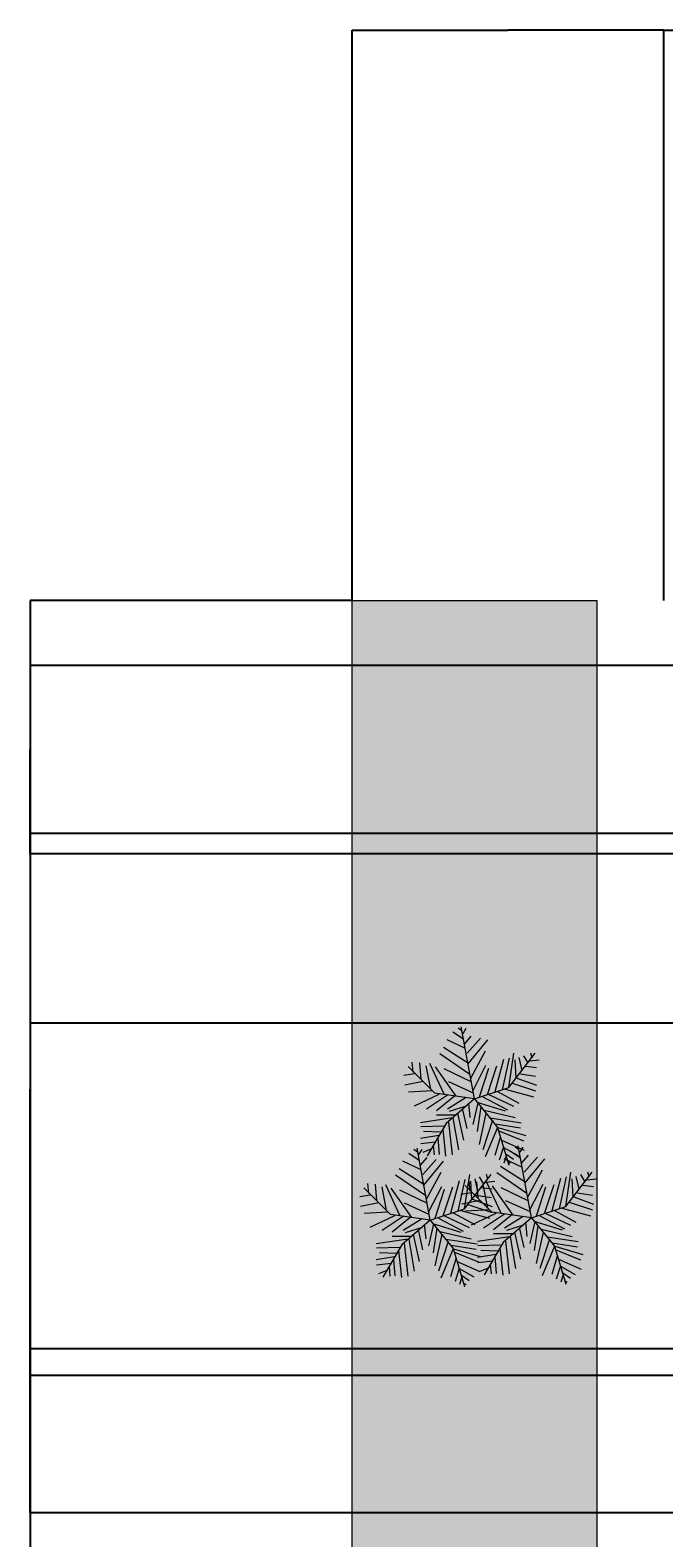
# Model space of a CAD drawing. Units: millimetres. Extents: x -229 to 16545, y -10488 to 4272.
# Tile 4 of 29: x -229 to 2016, y -1067 to 4272. Entities that reach past the tile are written whole.
import ezdxf

# ---------------------------------------------------------------- set-up
doc = ezdxf.new("R2010")
doc.units = ezdxf.units.MM
for name, color, linetype, lineweight in [('A-ANNO-DIMS', 2, 'Continuous', 18), ('L-PLNT-BEDS', 82, 'Continuous', 18), ('L-PLNT-TREE', 80, 'Continuous', 18)]:
    doc.layers.add(name, color=color, linetype=linetype, lineweight=lineweight)
doc.layers.add('L-PLNT-PATT', color=116, linetype='Continuous', lineweight=13, true_color=0x136734)
doc.styles.get("Standard").update_dxf_attribs({"font": 'arial.ttf'})
doc.dimstyles.get("Standard").update_dxf_attribs({"dimtxt": 0.18, "dimasz": 0.18, "dimexe": 0.18, "dimexo": 0.0625, "dimgap": 0.09, "dimtad": 0, "dimtih": 1, "dimtoh": 1, "dimdec": 4, "dimzin": 0, "dimdsep": 46, "dimtxsty": 'Standard', "dimcen": 0.09, "dimadec": 0, "dimazin": 0, "dimtfac": 1, "dimtdec": 4, "dimtofl": 0, "dimtmove": 0, "dimatfit": 3, "dimfxl": 1, "dimtolj": 1, "dimtzin": 0, "dimarcsym": 0})

# ---------------------------------------------------------------- blocks, each defined once
blk = doc.blocks.new('*U18')
for p, q in [((-8.737, 47.138), (-17.069, 52.711)), ((-10.186, 53.64), (-13.084, 55.962)), ((0, 0), (-10.5, 57)), ((-9.099, 51.782), (-6.563, 55.962)), ((-7.65, 43.423), (-2.578, 49.46)), ((-5.839, 35.992), (4.667, 48.067)), ((-5.114, 28.097), (-24.676, 40.636)), ((-7.288, 39.707), (-21.778, 46.673)), ((-5.114, 27.632), (10.463, 46.673)), ((-2.941, 16.486), (8.652, 37.85)), ((27, 9), (48, 36)), ((27.127, 9.056), (31.112, 35.992)), ((44.153, 36.456), (45.239, 32.741)), ((-31.5, 4.5), (-52.5, 25.5)), ((-48.585, 21.131), (-49.309, 29.026)), ((-43.513, 28.561), (-42.427, 15.558)), ((-38.442, 26.239), (-34.819, 7.663)), ((-35.544, 28.097), (-24.314, 3.947)), ((-14.533, 2.09), (-30.834, 25.31)), ((-3.665, 19.273), (-27.574, 35.527)), ((-24.314, 23.917), (-2.941, 13.7)), ((-1.129, 6.734), (9.014, 26.704)), ((3.942, 1.625), (11.187, 24.381)), ((10.101, 3.483), (17.708, 26.239)), ((16.259, 5.805), (23.142, 31.348)), ((22.055, 7.198), (27.489, 32.277)), ((31.836, 30.883), (32.561, 16.486)), ((35.096, 32.741), (37.27, 22.524)), ((38.719, 34.134), (41.979, 28.561)), ((40.53, 25.775), (48.862, 24.846)), ((43.791, 29.954), (51.036, 30.883)), ((-47.498, 19.737), (-55.83, 18.344)), ((-40.615, 13.7), (-55.105, 10.913)), ((-20.691, 13.7), (-1.129, 4.876)), ((29.662, 12.307), (48.137, 6.269)), ((33.285, 16.486), (48.862, 10.913)), ((36.183, 19.737), (48.137, 17.88)), ((-33.37, 6.269), (-52.207, 5.34)), ((-28.299, 3.483), (-47.86, -5.805)), ((-21.416, 3.018), (-38.079, -8.128)), ((0, 0), (-31.5, 4.5)), ((-15.982, 2.09), (-30.11, -9.521)), ((0, 0), (-22.5, -19.5)), ((-6.563, 1.161), (-21.416, -8.128)), ((0, 0), (27, 9)), ((0, 0), (18, -22.5)), ((6.478, 1.625), (26.04, -8.592)), ((11.187, 3.483), (30.749, -5.805)), ((18.07, 5.805), (35.096, -3.483)), ((24.229, 7.663), (46.688, 1.625)), ((-6.563, -5.805), (-19.967, -9.985)), ((-13.446, -11.378), (-8.737, -32.741)), ((-9.461, -8.592), (-6.201, -23.453)), ((-4.752, -3.483), (-3.665, -14.629)), ((2.493, -3.019), (-1.491, -20.202)), ((1.769, -2.555), (24.229, -9.521)), ((5.029, -6.27), (2.131, -25.775)), ((9.014, -11.378), (3.58, -35.992)), ((7.565, -9.056), (32.198, -14.629)), ((-17.431, -15.094), (-42.789, -18.809)), ((-24.314, -21.596), (-42.427, -22.06)), ((-22.5, -19.5), (-37.5, -45)), ((-15.257, -12.772), (-30.11, -12.772)), ((-20.691, -18.345), (-17.793, -44.352)), ((-17.069, -15.094), (-12.721, -40.172)), ((14.085, -16.951), (6.478, -40.172)), ((18.07, -22.524), (8.289, -45.745)), ((12.274, -15.094), (36.907, -18.809)), ((16.259, -19.738), (36.183, -22.989)), ((18, -22.5), (27, -52.5)), ((18.433, -22.524), (40.53, -29.026)), ((-28.299, -29.026), (-42.789, -31.348)), ((-30.834, -34.135), (-42.427, -35.528)), ((-26.849, -26.24), (-40.253, -25.775)), ((-29.023, -30.884), (-27.936, -43.887)), ((-25.038, -23.918), (-22.865, -45.281)), ((20.244, -30.419), (15.897, -44.816)), ((19.157, -25.311), (38.719, -33.206)), ((21.331, -32.741), (39.081, -40.636)), ((-34.457, -39.708), (-40.978, -42.494)), ((-32.646, -36.921), (-31.921, -44.352)), ((22.78, -37.85), (19.519, -48.532)), ((22.78, -38.314), (34.372, -44.816)), ((24.591, -45.745), (23.142, -50.854)), ((24.591, -43.423), (30.749, -47.603)), ((26.764, -49.925), (28.213, -50.854))]:
    blk.add_line(p, q)
blk = doc.blocks.new('*D45')
at = {"layer": 'A-ANNO-DIMS', "color": 0, "lineweight": -2, "transparency": 16777216}
for p, q in [((2015.9, 2251.8), (2015.9, 4271.7)), ((2016.1, 4271.5), (8015.5, 4271.5)), ((14015.8, 4271.5), (8016.4, 4271.5)), ((14015.9, 2251.8), (14015.9, 4271.7))]:
    blk.add_line(p, q, dxfattribs=at)
at = {"layer": 'A-ANNO-DIMS', "color": 0, "transparency": 16777216}
for points in [[(2016.1, 4271.5), (2016.1, 4271.4), (2015.9, 4271.5)], [(14015.8, 4271.5), (14015.8, 4271.4), (14015.9, 4271.5)]]:
    blk.add_solid(points, dxfattribs=at)
at = {"layer": 'Defpoints', "color": 0, "transparency": 16777216}
for p in [(14015.9, 4271.5), (2015.9, 2251.7), (14015.9, 2251.7)]:
    blk.add_point(p, dxfattribs=at)
at = {"layer": 'A-ANNO-DIMS', "color": 0, "transparency": 16777216, "insert": (8015.9, 4271.5), "char_height": 0.18, "attachment_point": 5}
blk.add_mtext('\\A1;12000', dxfattribs=at)
blk = doc.blocks.new('*D46')
at = {"layer": 'A-ANNO-DIMS', "color": 0, "lineweight": -2, "transparency": 16777216}
for p, q in [((912, 2251.7), (-228.8, 2251.7)), ((-228.7, 2251.5), (-228.7, -3498.1)), ((-228.7, -9248.1), (-228.7, -3498.5)), ((912, -9248.3), (-228.8, -9248.3))]:
    blk.add_line(p, q, dxfattribs=at)
at = {"layer": 'A-ANNO-DIMS', "color": 0, "transparency": 16777216}
for points in [[(-228.7, 2251.5), (-228.6, 2251.5), (-228.7, 2251.7)], [(-228.7, -9248.1), (-228.6, -9248.1), (-228.7, -9248.3)]]:
    blk.add_solid(points, dxfattribs=at)
at = {"layer": 'Defpoints', "color": 0, "transparency": 16777216}
for p in [(912.1, 2251.7), (-228.7, -9248.3), (912.1, -9248.3)]:
    blk.add_point(p, dxfattribs=at)
at = {"layer": 'A-ANNO-DIMS', "color": 0, "transparency": 16777216, "insert": (-228.7, -3498.3), "char_height": 0.18, "attachment_point": 5}
blk.add_mtext('\\A1;11500', dxfattribs=at)
blk = doc.blocks.new('*D49')
at = {"layer": 'A-ANNO-DIMS', "color": 0, "lineweight": -2, "transparency": 16777216}
for p, q in [((912.1, 2251.8), (912.1, 4271.7)), ((912.2, 4271.5), (1463.5, 4271.5)), ((2015.8, 4271.5), (1464.4, 4271.5)), ((2015.9, 2251.8), (2015.9, 4271.7))]:
    blk.add_line(p, q, dxfattribs=at)
at = {"layer": 'A-ANNO-DIMS', "color": 0, "transparency": 16777216}
for points in [[(912.2, 4271.5), (912.2, 4271.4), (912.1, 4271.5)], [(2015.8, 4271.5), (2015.8, 4271.4), (2015.9, 4271.5)]]:
    blk.add_solid(points, dxfattribs=at)
at = {"layer": 'Defpoints', "color": 0, "transparency": 16777216}
for p in [(2015.9, 4271.5), (912.1, 2251.7), (2015.9, 2251.7)]:
    blk.add_point(p, dxfattribs=at)
at = {"layer": 'A-ANNO-DIMS', "color": 0, "transparency": 16777216, "insert": (1464, 4271.5), "char_height": 0.18, "attachment_point": 5}
blk.add_mtext('\\A1;1103.9', dxfattribs=at)
blk = doc.blocks.new('*D53')
at = {"layer": 'A-ANNO-DIMS', "color": 0, "lineweight": -2, "transparency": 16777216}
for p, q in [((2245.9, 2021.7), (-228.8, 2021.7)), ((-228.7, 2021.5), (-228.7, 521.9)), ((-228.7, -978.1), (-228.7, 521.5)), ((2245.9, -978.3), (-228.8, -978.3))]:
    blk.add_line(p, q, dxfattribs=at)
at = {"layer": 'A-ANNO-DIMS', "color": 0, "transparency": 16777216}
for points in [[(-228.7, 2021.5), (-228.6, 2021.5), (-228.7, 2021.7)], [(-228.7, -978.1), (-228.6, -978.1), (-228.7, -978.3)]]:
    blk.add_solid(points, dxfattribs=at)
at = {"layer": 'Defpoints', "color": 0, "transparency": 16777216}
for p in [(2245.9, 2021.7), (-228.7, -978.3), (2245.9, -978.3)]:
    blk.add_point(p, dxfattribs=at)
at = {"layer": 'A-ANNO-DIMS', "color": 0, "transparency": 16777216, "insert": (-228.7, 521.7), "char_height": 0.18, "attachment_point": 5}
blk.add_mtext('\\A1;3000', dxfattribs=at)
blk = doc.blocks.new('*D64')
at = {"layer": 'A-ANNO-DIMS', "color": 0, "lineweight": -2, "transparency": 16777216}
for p, q in [((5745.9, 755.5), (-228.8, 755.5)), ((-228.7, 755.3), (-228.7, 179.2)), ((-228.7, -397.3), (-228.7, 178.8)), ((5745.9, -397.5), (-228.8, -397.5))]:
    blk.add_line(p, q, dxfattribs=at)
at = {"layer": 'A-ANNO-DIMS', "color": 0, "transparency": 16777216}
for points in [[(-228.7, 755.3), (-228.6, 755.3), (-228.7, 755.5)], [(-228.7, -397.3), (-228.6, -397.3), (-228.7, -397.5)]]:
    blk.add_solid(points, dxfattribs=at)
at = {"layer": 'Defpoints', "color": 0, "transparency": 16777216}
for p in [(5745.9, 755.5), (-228.7, -397.5), (5745.9, -397.5)]:
    blk.add_point(p, dxfattribs=at)
at = {"layer": 'A-ANNO-DIMS', "color": 0, "transparency": 16777216, "insert": (-228.7, 179), "char_height": 0.18, "attachment_point": 5}
blk.add_mtext('\\A1;1153', dxfattribs=at)
blk = doc.blocks.new('*D76')
at = {"layer": 'A-ANNO-DIMS', "color": 0, "lineweight": -2, "transparency": 16777216}
for p, q in [((5745.9, 2021.7), (-228.8, 2021.7)), ((-228.7, 2021.5), (-228.7, 1724.7)), ((-228.7, 1427.4), (-228.7, 1724.3)), ((5745.9, 1427.3), (-228.8, 1427.3))]:
    blk.add_line(p, q, dxfattribs=at)
at = {"layer": 'A-ANNO-DIMS', "color": 0, "transparency": 16777216}
for points in [[(-228.7, 2021.5), (-228.6, 2021.5), (-228.7, 2021.7)], [(-228.7, 1427.4), (-228.6, 1427.4), (-228.7, 1427.3)]]:
    blk.add_solid(points, dxfattribs=at)
at = {"layer": 'Defpoints', "color": 0, "transparency": 16777216}
for p in [(5745.9, 2021.7), (-228.7, 1427.3), (5745.9, 1427.3)]:
    blk.add_point(p, dxfattribs=at)
at = {"layer": 'A-ANNO-DIMS', "color": 0, "transparency": 16777216, "insert": (-228.7, 1724.5), "char_height": 0.18, "attachment_point": 5}
blk.add_mtext('\\A1;594.5', dxfattribs=at)
blk = doc.blocks.new('*D78')
at = {"layer": 'A-ANNO-DIMS', "color": 0, "lineweight": -2, "transparency": 16777216}
for p, q in [((5013.3, -492.9), (-228.8, -492.9)), ((-228.7, -493.1), (-228.7, -735.4)), ((-228.7, -978.1), (-228.7, -735.8)), ((5013.3, -978.3), (-228.8, -978.3))]:
    blk.add_line(p, q, dxfattribs=at)
at = {"layer": 'A-ANNO-DIMS', "color": 0, "transparency": 16777216}
for points in [[(-228.7, -493.1), (-228.6, -493.1), (-228.7, -492.9)], [(-228.7, -978.1), (-228.6, -978.1), (-228.7, -978.3)]]:
    blk.add_solid(points, dxfattribs=at)
at = {"layer": 'Defpoints', "color": 0, "transparency": 16777216}
for p in [(-228.7, -492.9), (5013.3, -492.9), (5013.3, -978.3)]:
    blk.add_point(p, dxfattribs=at)
at = {"layer": 'A-ANNO-DIMS', "color": 0, "transparency": 16777216, "insert": (-228.7, -735.6), "char_height": 0.18, "attachment_point": 5}
blk.add_mtext('\\A1;485.3', dxfattribs=at)
blk = doc.blocks.new('*D89')
at = {"layer": 'A-ANNO-DIMS', "color": 0, "lineweight": -2, "transparency": 16777216}
for p, q in [((5745.9, -397.5), (-228.8, -397.5)), ((-228.7, -397.7), (-228.7, -687.7)), ((-228.7, -978.1), (-228.7, -688.1)), ((5745.9, -978.3), (-228.8, -978.3))]:
    blk.add_line(p, q, dxfattribs=at)
at = {"layer": 'A-ANNO-DIMS', "color": 0, "transparency": 16777216}
for points in [[(-228.7, -397.7), (-228.6, -397.7), (-228.7, -397.5)], [(-228.7, -978.1), (-228.6, -978.1), (-228.7, -978.3)]]:
    blk.add_solid(points, dxfattribs=at)
at = {"layer": 'Defpoints', "color": 0, "transparency": 16777216}
for p in [(5745.9, -397.5), (-228.7, -978.3), (5745.9, -978.3)]:
    blk.add_point(p, dxfattribs=at)
at = {"layer": 'A-ANNO-DIMS', "color": 0, "transparency": 16777216, "insert": (-228.7, -687.9), "char_height": 0.18, "attachment_point": 5}
blk.add_mtext('\\A1;580.8', dxfattribs=at)
blk = doc.blocks.new('*D100')
at = {"layer": 'A-ANNO-DIMS', "color": 0, "lineweight": -2, "transparency": 16777216}
for p, q in [((7294.4, 2021.7), (-228.8, 2021.7)), ((-228.7, 2021.5), (-228.7, 1688.2)), ((-228.7, 1354.6), (-228.7, 1687.9)), ((8024.8, 1354.4), (-228.8, 1354.4))]:
    blk.add_line(p, q, dxfattribs=at)
at = {"layer": 'A-ANNO-DIMS', "color": 0, "transparency": 16777216}
for points in [[(-228.7, 2021.5), (-228.6, 2021.5), (-228.7, 2021.7)], [(-228.7, 1354.6), (-228.6, 1354.6), (-228.7, 1354.4)]]:
    blk.add_solid(points, dxfattribs=at)
at = {"layer": 'Defpoints', "color": 0, "transparency": 16777216}
for p in [(7294.4, 2021.7), (-228.7, 1354.4), (8024.9, 1354.4)]:
    blk.add_point(p, dxfattribs=at)
at = {"layer": 'A-ANNO-DIMS', "color": 0, "transparency": 16777216, "insert": (-228.7, 1688.1), "char_height": 0.18, "attachment_point": 5}
blk.add_mtext('\\A1;667.3', dxfattribs=at)

msp = doc.modelspace()

# ---------------------------------------------------------------- hatches: boundary and pattern name
at = {"layer": 'L-PLNT-PATT'}
h = msp.add_hatch(dxfattribs=at)
h.set_pattern_fill('GRASS', color=256)
h.set_pattern_definition([(90, (-8141.222, -13125.504), (-17.960512, 17.960512), [4.7625, -31.158524]), (45, (-8141.222, -13125.504), (-17.960512, 17.960512), [4.7625, -20.6375]), (135, (-8141.222, -13125.504), (-17.960512, -17.960512), [4.7625, -20.6375])])
h.paths.add_polyline_path([(1778.331, 2251.728), (912.052, 2251.728), (912.052, -9248.272), (1778.331, -9248.272), (1914.943, -9248.272), (1914.943, -7879.258), (1778.331, -7879.258)])
h = msp.add_hatch(dxfattribs=at)
h.set_pattern_fill('GRASS', color=256, scale=5.9)
h.set_pattern_definition([(90, (-8141.22, -13125.5), (-105.967, 105.967), [28.0987, -183.8353]), (45, (-8141.22, -13125.5), (-105.967, 105.967), [28.0987, -121.7613]), (135, (-8141.22, -13125.5), (-105.967, -105.967), [28.0987, -121.7613])])
h.paths.add_polyline_path([(1778.331, 2251.728), (912.052, 2251.728), (912.052, -9248.272), (1778.331, -9248.272), (1914.943, -9248.272), (1914.943, -7879.258), (1778.331, -7879.258)])

# ---------------------------------------------------------------- linework, layer by layer
at = {"layer": 'L-PLNT-BEDS', "transparency": 33554554}
for p, q in [((912.052, -9248.272), (912.052, 2251.728)), ((912.052, 2251.728), (1778.331, 2251.728))]:
    msp.add_line(p, q, dxfattribs=at)
at = {"layer": 'L-PLNT-BEDS', "transparency": 33554569}
msp.add_line((1778.331, 2251.728), (1778.331, -7879.258), dxfattribs=at)

# ---------------------------------------------------------------- block references
at = {"layer": 'L-PLNT-TREE', "xscale": 4.481031954380777, "yscale": 4.481031954380777, "zscale": 4.481031954380777}
for p in [(1345.416, 487.16), (1547.417, 65.913), (1188.67, 57.588)]:
    msp.add_blockref('*U18', p, dxfattribs=at)

# ---------------------------------------------------------------- dimensions: what is measured, and where the dimension line sits
at = {"layer": 'A-ANNO-DIMS'}
for base, p1, p2, override, picture, middle in [((2015.933, 4271.479), (912.052, 2251.728), (2015.933, 2251.728), {"dimdec": 1, "dimlfac": 1, "dimrnd": 0, "dimzin": 0, "dimdsep": 46, "dimlunit": 2}, '*D49', (1463.993, 4271.479)), ((14015.933, 4271.479), (2015.933, 2251.728), (14015.933, 2251.728), {"dimdec": 0, "dimlfac": 1, "dimrnd": 0, "dimzin": 0, "dimdsep": 46, "dimlunit": 2}, '*D45', (8015.933, 4271.479))]:
    dim = msp.add_linear_dim(base=base, p1=p1, p2=p2, dimstyle='Standard', override=override, dxfattribs=at)
    dim.commit()
    dim.dimension.update_dxf_attribs({"geometry": picture, "text_midpoint": middle})
for base, p1, p2, override, picture, middle in [((-228.657, -9248.272), (912.052, 2251.728), (912.052, -9248.272), {"dimdec": 0, "dimlfac": 1, "dimrnd": 0, "dimzin": 0, "dimdsep": 46, "dimlunit": 2}, '*D46', (-228.657, -3498.272)), ((-228.657, 1427.266), (5745.933, 2021.728), (5745.933, 1427.266), {"dimdec": 1, "dimlfac": 1, "dimrnd": 0, "dimzin": 0, "dimdsep": 46, "dimlunit": 2}, '*D76', (-228.657, 1724.497)), ((-228.657, 1354.386), (7294.425, 2021.728), (8024.889, 1354.386), {"dimdec": 1, "dimlfac": 1, "dimrnd": 0, "dimzin": 0, "dimdsep": 46, "dimlunit": 2}, '*D100', (-228.657, 1688.057)), ((-228.657, -978.272), (2245.933, 2021.728), (2245.933, -978.272), {"dimdec": 0, "dimlfac": 1, "dimrnd": 0, "dimzin": 0, "dimdsep": 46, "dimlunit": 2}, '*D53', (-228.657, 521.728)), ((-228.657, -397.513), (5745.933, 755.492), (5745.933, -397.513), {"dimdec": 0, "dimlfac": 1, "dimrnd": 0, "dimzin": 0, "dimdsep": 46, "dimlunit": 2}, '*D64', (-228.657, 178.99)), ((-228.657, -978.272), (5745.933, -397.513), (5745.933, -978.272), {"dimdec": 1, "dimlfac": 1, "dimrnd": 0, "dimzin": 0, "dimdsep": 46, "dimlunit": 2}, '*D89', (-228.657, -687.892)), ((-228.657, -492.942), (5013.319, -978.272), (5013.319, -492.942), {"dimdec": 1, "dimlfac": 1, "dimrnd": 0, "dimzin": 0, "dimdsep": 46, "dimlunit": 2}, '*D78', (-228.657, -735.607))]:
    dim = msp.add_linear_dim(base=base, p1=p1, p2=p2, angle=90, dimstyle='Standard', override=override, dxfattribs=at)
    dim.commit()
    dim.dimension.update_dxf_attribs({"geometry": picture, "text_midpoint": middle})

doc.saveas('drawing.dxf')
